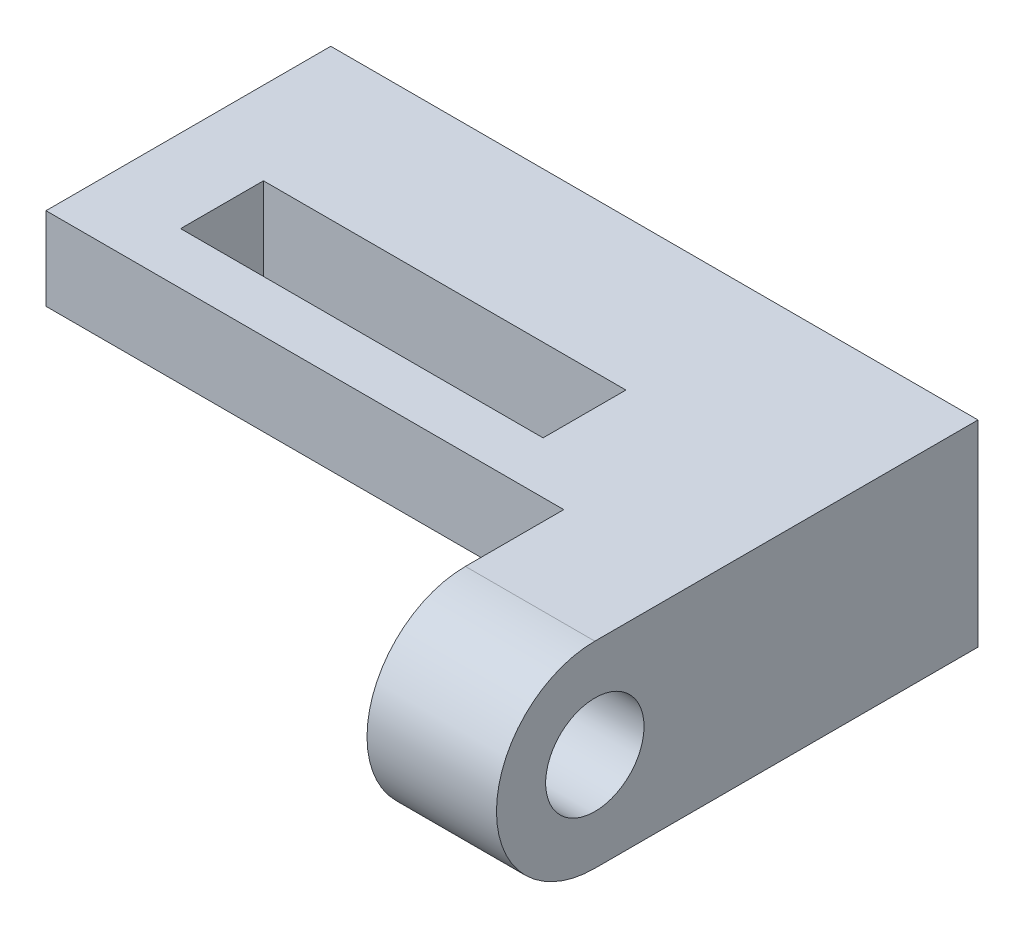
ISO-10303-21;
HEADER;
FILE_DESCRIPTION(('STEP AP214'),'2;1');
FILE_NAME('part.step','',(''),(''),'','','');
FILE_SCHEMA(('AUTOMOTIVE_DESIGN { 1 0 10303 214 1 1 1 1 }'));
ENDSEC;
DATA;
#1=APPLICATION_CONTEXT('core data for automotive mechanical design processes');
#2=APPLICATION_PROTOCOL_DEFINITION('international standard','automotive_design',2000,#1);
#3=PRODUCT_CONTEXT('',#1,'mechanical');
#4=PRODUCT('Part','Part','',(#3));
#5=PRODUCT_RELATED_PRODUCT_CATEGORY('part','',(#4));
#6=PRODUCT_DEFINITION_FORMATION('','',#4);
#7=PRODUCT_DEFINITION_CONTEXT('part definition',#1,'design');
#8=PRODUCT_DEFINITION('design','',#6,#7);
#9=PRODUCT_DEFINITION_SHAPE('','',#8);
#10=(LENGTH_UNIT() NAMED_UNIT(*) SI_UNIT(.MILLI.,.METRE.));
#11=(NAMED_UNIT(*) PLANE_ANGLE_UNIT() SI_UNIT($,.RADIAN.));
#12=(NAMED_UNIT(*) SI_UNIT($,.STERADIAN.) SOLID_ANGLE_UNIT());
#13=UNCERTAINTY_MEASURE_WITH_UNIT(LENGTH_MEASURE(1.E-05),#10,'distance_accuracy_value','');
#14=(GEOMETRIC_REPRESENTATION_CONTEXT(3) GLOBAL_UNCERTAINTY_ASSIGNED_CONTEXT((#13)) GLOBAL_UNIT_ASSIGNED_CONTEXT((#10,
#11,#12)) REPRESENTATION_CONTEXT('',''));
#15=CARTESIAN_POINT('',(0.,0.,0.));
#16=DIRECTION('',(0.,0.,1.));
#17=DIRECTION('',(1.,0.,0.));
#18=AXIS2_PLACEMENT_3D('',#15,#16,#17);
#19=CARTESIAN_POINT('',(0.,0.,10.));
#20=DIRECTION('',(0.,0.,1.));
#21=DIRECTION('',(1.,0.,0.));
#22=AXIS2_PLACEMENT_3D('',#19,#20,#21);
#23=PLANE('',#22);
#24=CARTESIAN_POINT('',(25.,13.,10.));
#25=DIRECTION('',(0.,0.,1.));
#26=DIRECTION('',(1.,0.,0.));
#27=AXIS2_PLACEMENT_3D('',#24,#25,#26);
#28=CIRCLE('',#27,6.5);
#29=CARTESIAN_POINT('',(31.5,13.,10.));
#30=VERTEX_POINT('',#29);
#31=EDGE_CURVE('E501',#30,#30,#28,.T.);
#32=ORIENTED_EDGE('',*,*,#31,.F.);
#33=EDGE_LOOP('',(#32));
#34=FACE_BOUND('',#33,.T.);
#35=CARTESIAN_POINT('',(75.,13.,10.));
#36=DIRECTION('',(0.,0.,1.));
#37=DIRECTION('',(1.,0.,0.));
#38=AXIS2_PLACEMENT_3D('',#35,#36,#37);
#39=CIRCLE('',#38,6.5);
#40=CARTESIAN_POINT('',(81.5,13.,10.));
#41=VERTEX_POINT('',#40);
#42=EDGE_CURVE('E157',#41,#41,#39,.T.);
#43=ORIENTED_EDGE('',*,*,#42,.F.);
#44=EDGE_LOOP('',(#43));
#45=FACE_BOUND('',#44,.T.);
#46=DIRECTION('',(0.,1.,0.));
#47=VECTOR('',#46,1.);
#48=CARTESIAN_POINT('',(100.,0.,10.));
#49=LINE('',#48,#47);
#50=CARTESIAN_POINT('',(100.,0.,10.));
#51=VERTEX_POINT('',#50);
#52=CARTESIAN_POINT('',(100.,22.,10.));
#53=VERTEX_POINT('',#52);
#54=EDGE_CURVE('E199',#51,#53,#49,.T.);
#55=ORIENTED_EDGE('',*,*,#54,.T.);
#56=DIRECTION('',(-1.,0.,0.));
#57=VECTOR('',#56,1.);
#58=CARTESIAN_POINT('',(100.,22.,10.));
#59=LINE('',#58,#57);
#60=CARTESIAN_POINT('',(0.,22.,10.));
#61=VERTEX_POINT('',#60);
#62=EDGE_CURVE('E174',#53,#61,#59,.T.);
#63=ORIENTED_EDGE('',*,*,#62,.T.);
#64=DIRECTION('',(0.,-1.,0.));
#65=VECTOR('',#64,1.);
#66=CARTESIAN_POINT('',(0.,38.,10.));
#67=LINE('',#66,#65);
#68=CARTESIAN_POINT('',(0.,0.,10.));
#69=VERTEX_POINT('',#68);
#70=EDGE_CURVE('E219',#61,#69,#67,.T.);
#71=ORIENTED_EDGE('',*,*,#70,.T.);
#72=DIRECTION('',(1.,0.,0.));
#73=VECTOR('',#72,1.);
#74=CARTESIAN_POINT('',(0.,0.,10.));
#75=LINE('',#74,#73);
#76=EDGE_CURVE('E224',#69,#51,#75,.T.);
#77=ORIENTED_EDGE('',*,*,#76,.T.);
#78=EDGE_LOOP('',(#55,#63,#71,#77));
#79=FACE_BOUND('',#78,.T.);
#80=ADVANCED_FACE('F44',(#34,#45,#79),#23,.T.);
#81=CARTESIAN_POINT('',(0.,38.,10.));
#82=DIRECTION('',(1.,0.,0.));
#83=DIRECTION('',(0.,0.,-1.));
#84=AXIS2_PLACEMENT_3D('',#81,#82,#83);
#85=PLANE('',#84);
#86=DIRECTION('',(0.,-1.,0.));
#87=VECTOR('',#86,1.);
#88=CARTESIAN_POINT('',(0.,38.,0.));
#89=LINE('',#88,#87);
#90=CARTESIAN_POINT('',(0.,38.,0.));
#91=VERTEX_POINT('',#90);
#92=CARTESIAN_POINT('',(0.,0.,0.));
#93=VERTEX_POINT('',#92);
#94=EDGE_CURVE('E220',#91,#93,#89,.T.);
#95=ORIENTED_EDGE('',*,*,#94,.T.);
#96=DIRECTION('',(0.,0.,-1.));
#97=VECTOR('',#96,1.);
#98=CARTESIAN_POINT('',(0.,0.,10.));
#99=LINE('',#98,#97);
#100=EDGE_CURVE('E11',#69,#93,#99,.T.);
#101=ORIENTED_EDGE('',*,*,#100,.F.);
#102=ORIENTED_EDGE('',*,*,#70,.F.);
#103=DIRECTION('',(0.,0.,1.));
#104=VECTOR('',#103,1.);
#105=CARTESIAN_POINT('',(0.,22.,10.));
#106=LINE('',#105,#104);
#107=CARTESIAN_POINT('',(0.,22.,55.));
#108=VERTEX_POINT('',#107);
#109=EDGE_CURVE('E178',#61,#108,#106,.T.);
#110=ORIENTED_EDGE('',*,*,#109,.T.);
#111=DIRECTION('',(0.,1.,0.));
#112=VECTOR('',#111,1.);
#113=CARTESIAN_POINT('',(0.,22.,55.));
#114=LINE('',#113,#112);
#115=CARTESIAN_POINT('',(0.,38.,55.));
#116=VERTEX_POINT('',#115);
#117=EDGE_CURVE('E187',#108,#116,#114,.T.);
#118=ORIENTED_EDGE('',*,*,#117,.T.);
#119=DIRECTION('',(0.,0.,-1.));
#120=VECTOR('',#119,1.);
#121=CARTESIAN_POINT('',(0.,38.,10.));
#122=LINE('',#121,#120);
#123=EDGE_CURVE('E228',#116,#91,#122,.T.);
#124=ORIENTED_EDGE('',*,*,#123,.T.);
#125=EDGE_LOOP('',(#95,#101,#102,#110,#118,#124));
#126=FACE_BOUND('',#125,.T.);
#127=ADVANCED_FACE('F50',(#126),#85,.F.);
#128=CARTESIAN_POINT('',(0.,0.,10.));
#129=DIRECTION('',(0.,1.,0.));
#130=DIRECTION('',(0.,0.,1.));
#131=AXIS2_PLACEMENT_3D('',#128,#129,#130);
#132=PLANE('',#131);
#133=DIRECTION('',(1.,0.,0.));
#134=VECTOR('',#133,1.);
#135=CARTESIAN_POINT('',(0.,0.,0.));
#136=LINE('',#135,#134);
#137=CARTESIAN_POINT('',(125.,0.,0.));
#138=VERTEX_POINT('',#137);
#139=EDGE_CURVE('E230',#93,#138,#136,.T.);
#140=ORIENTED_EDGE('',*,*,#139,.T.);
#141=DIRECTION('',(0.,0.,-1.));
#142=VECTOR('',#141,1.);
#143=CARTESIAN_POINT('',(125.,0.,10.));
#144=LINE('',#143,#142);
#145=CARTESIAN_POINT('',(125.,0.,74.));
#146=VERTEX_POINT('',#145);
#147=EDGE_CURVE('E52',#146,#138,#144,.T.);
#148=ORIENTED_EDGE('',*,*,#147,.F.);
#149=DIRECTION('',(1.,0.,0.));
#150=VECTOR('',#149,1.);
#151=CARTESIAN_POINT('',(100.,0.,74.));
#152=LINE('',#151,#150);
#153=CARTESIAN_POINT('',(100.,0.,74.));
#154=VERTEX_POINT('',#153);
#155=EDGE_CURVE('E211',#154,#146,#152,.T.);
#156=ORIENTED_EDGE('',*,*,#155,.F.);
#157=DIRECTION('',(0.,0.,-1.));
#158=VECTOR('',#157,1.);
#159=CARTESIAN_POINT('',(100.,0.,74.));
#160=LINE('',#159,#158);
#161=EDGE_CURVE('E206',#154,#51,#160,.T.);
#162=ORIENTED_EDGE('',*,*,#161,.T.);
#163=ORIENTED_EDGE('',*,*,#76,.F.);
#164=ORIENTED_EDGE('',*,*,#100,.T.);
#165=EDGE_LOOP('',(#140,#148,#156,#162,#163,#164));
#166=FACE_BOUND('',#165,.T.);
#167=ADVANCED_FACE('F269',(#166),#132,.F.);
#168=CARTESIAN_POINT('',(125.,0.,10.));
#169=DIRECTION('',(-1.,0.,0.));
#170=DIRECTION('',(0.,0.,1.));
#171=AXIS2_PLACEMENT_3D('',#168,#169,#170);
#172=PLANE('',#171);
#173=CARTESIAN_POINT('',(125.,19.,74.));
#174=DIRECTION('',(1.,0.,0.));
#175=DIRECTION('',(0.,0.,-1.));
#176=AXIS2_PLACEMENT_3D('',#173,#174,#175);
#177=CIRCLE('',#176,9.5);
#178=CARTESIAN_POINT('',(125.,19.,64.5));
#179=VERTEX_POINT('',#178);
#180=EDGE_CURVE('E192',#179,#179,#177,.T.);
#181=ORIENTED_EDGE('',*,*,#180,.F.);
#182=EDGE_LOOP('',(#181));
#183=FACE_BOUND('',#182,.T.);
#184=DIRECTION('',(0.,1.,0.));
#185=VECTOR('',#184,1.);
#186=CARTESIAN_POINT('',(125.,0.,0.));
#187=LINE('',#186,#185);
#188=CARTESIAN_POINT('',(125.,38.,0.));
#189=VERTEX_POINT('',#188);
#190=EDGE_CURVE('E233',#138,#189,#187,.T.);
#191=ORIENTED_EDGE('',*,*,#190,.T.);
#192=DIRECTION('',(0.,0.,-1.));
#193=VECTOR('',#192,1.);
#194=CARTESIAN_POINT('',(125.,38.,10.));
#195=LINE('',#194,#193);
#196=CARTESIAN_POINT('',(125.,38.,74.));
#197=VERTEX_POINT('',#196);
#198=EDGE_CURVE('E236',#197,#189,#195,.T.);
#199=ORIENTED_EDGE('',*,*,#198,.F.);
#200=CARTESIAN_POINT('',(125.,19.,74.));
#201=DIRECTION('',(1.,0.,0.));
#202=DIRECTION('',(0.,0.,-1.));
#203=AXIS2_PLACEMENT_3D('',#200,#201,#202);
#204=CIRCLE('',#203,19.);
#205=EDGE_CURVE('E200',#197,#146,#204,.T.);
#206=ORIENTED_EDGE('',*,*,#205,.T.);
#207=ORIENTED_EDGE('',*,*,#147,.T.);
#208=EDGE_LOOP('',(#191,#199,#206,#207));
#209=FACE_BOUND('',#208,.T.);
#210=ADVANCED_FACE('F241',(#183,#209),#172,.F.);
#211=CARTESIAN_POINT('',(125.,38.,10.));
#212=DIRECTION('',(0.,-1.,0.));
#213=DIRECTION('',(0.,0.,-1.));
#214=AXIS2_PLACEMENT_3D('',#211,#212,#213);
#215=PLANE('',#214);
#216=DIRECTION('',(1.,0.,0.));
#217=VECTOR('',#216,1.);
#218=CARTESIAN_POINT('',(16.,38.,45.));
#219=LINE('',#218,#217);
#220=CARTESIAN_POINT('',(16.,38.,45.));
#221=VERTEX_POINT('',#220);
#222=CARTESIAN_POINT('',(86.,38.,45.));
#223=VERTEX_POINT('',#222);
#224=EDGE_CURVE('E165',#221,#223,#219,.T.);
#225=ORIENTED_EDGE('',*,*,#224,.F.);
#226=DIRECTION('',(0.,0.,1.));
#227=VECTOR('',#226,1.);
#228=CARTESIAN_POINT('',(16.,38.,29.));
#229=LINE('',#228,#227);
#230=CARTESIAN_POINT('',(16.,38.,29.));
#231=VERTEX_POINT('',#230);
#232=EDGE_CURVE('E58',#231,#221,#229,.T.);
#233=ORIENTED_EDGE('',*,*,#232,.F.);
#234=DIRECTION('',(-1.,0.,0.));
#235=VECTOR('',#234,1.);
#236=CARTESIAN_POINT('',(16.,38.,29.));
#237=LINE('',#236,#235);
#238=CARTESIAN_POINT('',(86.,38.,29.));
#239=VERTEX_POINT('',#238);
#240=EDGE_CURVE('E155',#239,#231,#237,.T.);
#241=ORIENTED_EDGE('',*,*,#240,.F.);
#242=DIRECTION('',(0.,0.,-1.));
#243=VECTOR('',#242,1.);
#244=CARTESIAN_POINT('',(86.,38.,29.));
#245=LINE('',#244,#243);
#246=EDGE_CURVE('E154',#223,#239,#245,.T.);
#247=ORIENTED_EDGE('',*,*,#246,.F.);
#248=EDGE_LOOP('',(#225,#233,#241,#247));
#249=FACE_BOUND('',#248,.T.);
#250=ORIENTED_EDGE('',*,*,#123,.F.);
#251=DIRECTION('',(1.,0.,0.));
#252=VECTOR('',#251,1.);
#253=CARTESIAN_POINT('',(0.,38.,55.));
#254=LINE('',#253,#252);
#255=CARTESIAN_POINT('',(100.,38.,55.));
#256=VERTEX_POINT('',#255);
#257=EDGE_CURVE('E171',#116,#256,#254,.T.);
#258=ORIENTED_EDGE('',*,*,#257,.T.);
#259=DIRECTION('',(0.,0.,1.));
#260=VECTOR('',#259,1.);
#261=CARTESIAN_POINT('',(100.,38.,10.));
#262=LINE('',#261,#260);
#263=CARTESIAN_POINT('',(100.,38.,74.));
#264=VERTEX_POINT('',#263);
#265=EDGE_CURVE('E202',#256,#264,#262,.T.);
#266=ORIENTED_EDGE('',*,*,#265,.T.);
#267=DIRECTION('',(1.,0.,0.));
#268=VECTOR('',#267,1.);
#269=CARTESIAN_POINT('',(100.,38.,74.));
#270=LINE('',#269,#268);
#271=EDGE_CURVE('E212',#264,#197,#270,.T.);
#272=ORIENTED_EDGE('',*,*,#271,.T.);
#273=ORIENTED_EDGE('',*,*,#198,.T.);
#274=DIRECTION('',(-1.,0.,0.));
#275=VECTOR('',#274,1.);
#276=CARTESIAN_POINT('',(125.,38.,0.));
#277=LINE('',#276,#275);
#278=EDGE_CURVE('E222',#189,#91,#277,.T.);
#279=ORIENTED_EDGE('',*,*,#278,.T.);
#280=EDGE_LOOP('',(#250,#258,#266,#272,#273,#279));
#281=FACE_BOUND('',#280,.T.);
#282=ADVANCED_FACE('F248',(#249,#281),#215,.F.);
#283=CARTESIAN_POINT('',(0.,0.,0.));
#284=DIRECTION('',(0.,0.,1.));
#285=DIRECTION('',(1.,0.,0.));
#286=AXIS2_PLACEMENT_3D('',#283,#284,#285);
#287=PLANE('',#286);
#288=CARTESIAN_POINT('',(25.,13.,0.));
#289=DIRECTION('',(0.,0.,1.));
#290=DIRECTION('',(1.,0.,0.));
#291=AXIS2_PLACEMENT_3D('',#288,#289,#290);
#292=CIRCLE('',#291,6.5);
#293=CARTESIAN_POINT('',(31.5,13.,0.));
#294=VERTEX_POINT('',#293);
#295=EDGE_CURVE('E164',#294,#294,#292,.T.);
#296=ORIENTED_EDGE('',*,*,#295,.T.);
#297=EDGE_LOOP('',(#296));
#298=FACE_BOUND('',#297,.T.);
#299=CARTESIAN_POINT('',(75.,13.,0.));
#300=DIRECTION('',(0.,0.,1.));
#301=DIRECTION('',(1.,0.,0.));
#302=AXIS2_PLACEMENT_3D('',#299,#300,#301);
#303=CIRCLE('',#302,6.5);
#304=CARTESIAN_POINT('',(81.5,13.,0.));
#305=VERTEX_POINT('',#304);
#306=EDGE_CURVE('E505',#305,#305,#303,.T.);
#307=ORIENTED_EDGE('',*,*,#306,.T.);
#308=EDGE_LOOP('',(#307));
#309=FACE_BOUND('',#308,.T.);
#310=ORIENTED_EDGE('',*,*,#94,.F.);
#311=ORIENTED_EDGE('',*,*,#278,.F.);
#312=ORIENTED_EDGE('',*,*,#190,.F.);
#313=ORIENTED_EDGE('',*,*,#139,.F.);
#314=EDGE_LOOP('',(#310,#311,#312,#313));
#315=FACE_BOUND('',#314,.T.);
#316=ADVANCED_FACE('F250',(#298,#309,#315),#287,.F.);
#317=CARTESIAN_POINT('',(100.,19.,74.));
#318=DIRECTION('',(1.,0.,0.));
#319=DIRECTION('',(0.,0.,-1.));
#320=AXIS2_PLACEMENT_3D('',#317,#318,#319);
#321=CYLINDRICAL_SURFACE('',#320,19.);
#322=ORIENTED_EDGE('',*,*,#205,.F.);
#323=ORIENTED_EDGE('',*,*,#271,.F.);
#324=CARTESIAN_POINT('',(100.,19.,74.));
#325=DIRECTION('',(1.,0.,0.));
#326=DIRECTION('',(0.,0.,-1.));
#327=AXIS2_PLACEMENT_3D('',#324,#325,#326);
#328=CIRCLE('',#327,19.);
#329=EDGE_CURVE('E201',#264,#154,#328,.T.);
#330=ORIENTED_EDGE('',*,*,#329,.T.);
#331=ORIENTED_EDGE('',*,*,#155,.T.);
#332=EDGE_LOOP('',(#322,#323,#330,#331));
#333=FACE_BOUND('',#332,.T.);
#334=ADVANCED_FACE('F262',(#333),#321,.T.);
#335=CARTESIAN_POINT('',(100.,19.,74.));
#336=DIRECTION('',(1.,0.,0.));
#337=DIRECTION('',(0.,0.,-1.));
#338=AXIS2_PLACEMENT_3D('',#335,#336,#337);
#339=PLANE('',#338);
#340=CARTESIAN_POINT('',(100.,19.,74.));
#341=DIRECTION('',(1.,0.,0.));
#342=DIRECTION('',(0.,0.,-1.));
#343=AXIS2_PLACEMENT_3D('',#340,#341,#342);
#344=CIRCLE('',#343,9.5);
#345=CARTESIAN_POINT('',(100.,19.,64.5));
#346=VERTEX_POINT('',#345);
#347=EDGE_CURVE('E191',#346,#346,#344,.T.);
#348=ORIENTED_EDGE('',*,*,#347,.T.);
#349=EDGE_LOOP('',(#348));
#350=FACE_BOUND('',#349,.T.);
#351=ORIENTED_EDGE('',*,*,#265,.F.);
#352=DIRECTION('',(0.,1.,0.));
#353=VECTOR('',#352,1.);
#354=CARTESIAN_POINT('',(100.,22.,55.));
#355=LINE('',#354,#353);
#356=CARTESIAN_POINT('',(100.,22.,55.));
#357=VERTEX_POINT('',#356);
#358=EDGE_CURVE('E189',#357,#256,#355,.T.);
#359=ORIENTED_EDGE('',*,*,#358,.F.);
#360=DIRECTION('',(0.,0.,-1.));
#361=VECTOR('',#360,1.);
#362=CARTESIAN_POINT('',(100.,22.,55.));
#363=LINE('',#362,#361);
#364=EDGE_CURVE('E182',#357,#53,#363,.T.);
#365=ORIENTED_EDGE('',*,*,#364,.T.);
#366=ORIENTED_EDGE('',*,*,#54,.F.);
#367=ORIENTED_EDGE('',*,*,#161,.F.);
#368=ORIENTED_EDGE('',*,*,#329,.F.);
#369=EDGE_LOOP('',(#351,#359,#365,#366,#367,#368));
#370=FACE_BOUND('',#369,.T.);
#371=ADVANCED_FACE('F264',(#350,#370),#339,.F.);
#372=CARTESIAN_POINT('',(100.,19.,74.));
#373=DIRECTION('',(1.,0.,0.));
#374=DIRECTION('',(0.,0.,-1.));
#375=AXIS2_PLACEMENT_3D('',#372,#373,#374);
#376=CYLINDRICAL_SURFACE('',#375,9.5);
#377=ORIENTED_EDGE('',*,*,#347,.F.);
#378=EDGE_LOOP('',(#377));
#379=FACE_BOUND('',#378,.T.);
#380=ORIENTED_EDGE('',*,*,#180,.T.);
#381=EDGE_LOOP('',(#380));
#382=FACE_BOUND('',#381,.T.);
#383=ADVANCED_FACE('F279',(#379,#382),#376,.F.);
#384=CARTESIAN_POINT('',(0.,22.,55.));
#385=DIRECTION('',(0.,0.,1.));
#386=DIRECTION('',(1.,0.,0.));
#387=AXIS2_PLACEMENT_3D('',#384,#385,#386);
#388=PLANE('',#387);
#389=ORIENTED_EDGE('',*,*,#257,.F.);
#390=ORIENTED_EDGE('',*,*,#117,.F.);
#391=DIRECTION('',(1.,0.,0.));
#392=VECTOR('',#391,1.);
#393=CARTESIAN_POINT('',(0.,22.,55.));
#394=LINE('',#393,#392);
#395=EDGE_CURVE('E181',#108,#357,#394,.T.);
#396=ORIENTED_EDGE('',*,*,#395,.T.);
#397=ORIENTED_EDGE('',*,*,#358,.T.);
#398=EDGE_LOOP('',(#389,#390,#396,#397));
#399=FACE_BOUND('',#398,.T.);
#400=ADVANCED_FACE('F257',(#399),#388,.T.);
#401=CARTESIAN_POINT('',(0.,22.,0.));
#402=DIRECTION('',(0.,1.,0.));
#403=DIRECTION('',(0.,0.,1.));
#404=AXIS2_PLACEMENT_3D('',#401,#402,#403);
#405=PLANE('',#404);
#406=DIRECTION('',(-1.,0.,0.));
#407=VECTOR('',#406,1.);
#408=CARTESIAN_POINT('',(16.,22.,29.));
#409=LINE('',#408,#407);
#410=CARTESIAN_POINT('',(86.,22.,29.));
#411=VERTEX_POINT('',#410);
#412=CARTESIAN_POINT('',(16.,22.,29.));
#413=VERTEX_POINT('',#412);
#414=EDGE_CURVE('E145',#411,#413,#409,.T.);
#415=ORIENTED_EDGE('',*,*,#414,.T.);
#416=DIRECTION('',(0.,0.,1.));
#417=VECTOR('',#416,1.);
#418=CARTESIAN_POINT('',(16.,22.,29.));
#419=LINE('',#418,#417);
#420=CARTESIAN_POINT('',(16.,22.,45.));
#421=VERTEX_POINT('',#420);
#422=EDGE_CURVE('E138',#413,#421,#419,.T.);
#423=ORIENTED_EDGE('',*,*,#422,.T.);
#424=DIRECTION('',(1.,0.,0.));
#425=VECTOR('',#424,1.);
#426=CARTESIAN_POINT('',(16.,22.,45.));
#427=LINE('',#426,#425);
#428=CARTESIAN_POINT('',(86.,22.,45.));
#429=VERTEX_POINT('',#428);
#430=EDGE_CURVE('E143',#421,#429,#427,.T.);
#431=ORIENTED_EDGE('',*,*,#430,.T.);
#432=DIRECTION('',(0.,0.,-1.));
#433=VECTOR('',#432,1.);
#434=CARTESIAN_POINT('',(86.,22.,29.));
#435=LINE('',#434,#433);
#436=EDGE_CURVE('E67',#429,#411,#435,.T.);
#437=ORIENTED_EDGE('',*,*,#436,.T.);
#438=EDGE_LOOP('',(#415,#423,#431,#437));
#439=FACE_BOUND('',#438,.T.);
#440=ORIENTED_EDGE('',*,*,#62,.F.);
#441=ORIENTED_EDGE('',*,*,#364,.F.);
#442=ORIENTED_EDGE('',*,*,#395,.F.);
#443=ORIENTED_EDGE('',*,*,#109,.F.);
#444=EDGE_LOOP('',(#440,#441,#442,#443));
#445=FACE_BOUND('',#444,.T.);
#446=ADVANCED_FACE('F146',(#439,#445),#405,.F.);
#447=CARTESIAN_POINT('',(16.,22.,29.));
#448=DIRECTION('',(-1.,0.,0.));
#449=DIRECTION('',(0.,0.,1.));
#450=AXIS2_PLACEMENT_3D('',#447,#448,#449);
#451=PLANE('',#450);
#452=ORIENTED_EDGE('',*,*,#232,.T.);
#453=DIRECTION('',(0.,1.,0.));
#454=VECTOR('',#453,1.);
#455=CARTESIAN_POINT('',(16.,22.,45.));
#456=LINE('',#455,#454);
#457=EDGE_CURVE('E135',#421,#221,#456,.T.);
#458=ORIENTED_EDGE('',*,*,#457,.F.);
#459=ORIENTED_EDGE('',*,*,#422,.F.);
#460=DIRECTION('',(0.,1.,0.));
#461=VECTOR('',#460,1.);
#462=CARTESIAN_POINT('',(16.,22.,29.));
#463=LINE('',#462,#461);
#464=EDGE_CURVE('E169',#413,#231,#463,.T.);
#465=ORIENTED_EDGE('',*,*,#464,.T.);
#466=EDGE_LOOP('',(#452,#458,#459,#465));
#467=FACE_BOUND('',#466,.T.);
#468=ADVANCED_FACE('F133',(#467),#451,.F.);
#469=CARTESIAN_POINT('',(16.,22.,29.));
#470=DIRECTION('',(0.,0.,-1.));
#471=DIRECTION('',(-1.,0.,0.));
#472=AXIS2_PLACEMENT_3D('',#469,#470,#471);
#473=PLANE('',#472);
#474=ORIENTED_EDGE('',*,*,#240,.T.);
#475=ORIENTED_EDGE('',*,*,#464,.F.);
#476=ORIENTED_EDGE('',*,*,#414,.F.);
#477=DIRECTION('',(0.,1.,0.));
#478=VECTOR('',#477,1.);
#479=CARTESIAN_POINT('',(86.,22.,29.));
#480=LINE('',#479,#478);
#481=EDGE_CURVE('E175',#411,#239,#480,.T.);
#482=ORIENTED_EDGE('',*,*,#481,.T.);
#483=EDGE_LOOP('',(#474,#475,#476,#482));
#484=FACE_BOUND('',#483,.T.);
#485=ADVANCED_FACE('F277',(#484),#473,.F.);
#486=CARTESIAN_POINT('',(86.,22.,29.));
#487=DIRECTION('',(1.,0.,0.));
#488=DIRECTION('',(0.,0.,-1.));
#489=AXIS2_PLACEMENT_3D('',#486,#487,#488);
#490=PLANE('',#489);
#491=ORIENTED_EDGE('',*,*,#246,.T.);
#492=ORIENTED_EDGE('',*,*,#481,.F.);
#493=ORIENTED_EDGE('',*,*,#436,.F.);
#494=DIRECTION('',(0.,1.,0.));
#495=VECTOR('',#494,1.);
#496=CARTESIAN_POINT('',(86.,22.,45.));
#497=LINE('',#496,#495);
#498=EDGE_CURVE('E142',#429,#223,#497,.T.);
#499=ORIENTED_EDGE('',*,*,#498,.T.);
#500=EDGE_LOOP('',(#491,#492,#493,#499));
#501=FACE_BOUND('',#500,.T.);
#502=ADVANCED_FACE('F392',(#501),#490,.F.);
#503=CARTESIAN_POINT('',(16.,22.,45.));
#504=DIRECTION('',(0.,0.,1.));
#505=DIRECTION('',(1.,0.,0.));
#506=AXIS2_PLACEMENT_3D('',#503,#504,#505);
#507=PLANE('',#506);
#508=ORIENTED_EDGE('',*,*,#224,.T.);
#509=ORIENTED_EDGE('',*,*,#498,.F.);
#510=ORIENTED_EDGE('',*,*,#430,.F.);
#511=ORIENTED_EDGE('',*,*,#457,.T.);
#512=EDGE_LOOP('',(#508,#509,#510,#511));
#513=FACE_BOUND('',#512,.T.);
#514=ADVANCED_FACE('F147',(#513),#507,.F.);
#515=CARTESIAN_POINT('',(75.,13.,0.));
#516=DIRECTION('',(0.,0.,1.));
#517=DIRECTION('',(1.,0.,0.));
#518=AXIS2_PLACEMENT_3D('',#515,#516,#517);
#519=CYLINDRICAL_SURFACE('',#518,6.5);
#520=ORIENTED_EDGE('',*,*,#306,.F.);
#521=EDGE_LOOP('',(#520));
#522=FACE_BOUND('',#521,.T.);
#523=ORIENTED_EDGE('',*,*,#42,.T.);
#524=EDGE_LOOP('',(#523));
#525=FACE_BOUND('',#524,.T.);
#526=ADVANCED_FACE('F418',(#522,#525),#519,.F.);
#527=CARTESIAN_POINT('',(25.,13.,0.));
#528=DIRECTION('',(0.,0.,1.));
#529=DIRECTION('',(1.,0.,0.));
#530=AXIS2_PLACEMENT_3D('',#527,#528,#529);
#531=CYLINDRICAL_SURFACE('',#530,6.5);
#532=ORIENTED_EDGE('',*,*,#295,.F.);
#533=EDGE_LOOP('',(#532));
#534=FACE_BOUND('',#533,.T.);
#535=ORIENTED_EDGE('',*,*,#31,.T.);
#536=EDGE_LOOP('',(#535));
#537=FACE_BOUND('',#536,.T.);
#538=ADVANCED_FACE('F437',(#534,#537),#531,.F.);
#539=CLOSED_SHELL('',(#80,#127,#167,#210,#282,#316,#334,#371,#383,#400,#446,#468,#485,#502,#514,
#526,#538));
#540=MANIFOLD_SOLID_BREP('B2',#539);
#541=ADVANCED_BREP_SHAPE_REPRESENTATION('',(#18,#540),#14);
#542=SHAPE_DEFINITION_REPRESENTATION(#9,#541);
ENDSEC;
END-ISO-10303-21;
